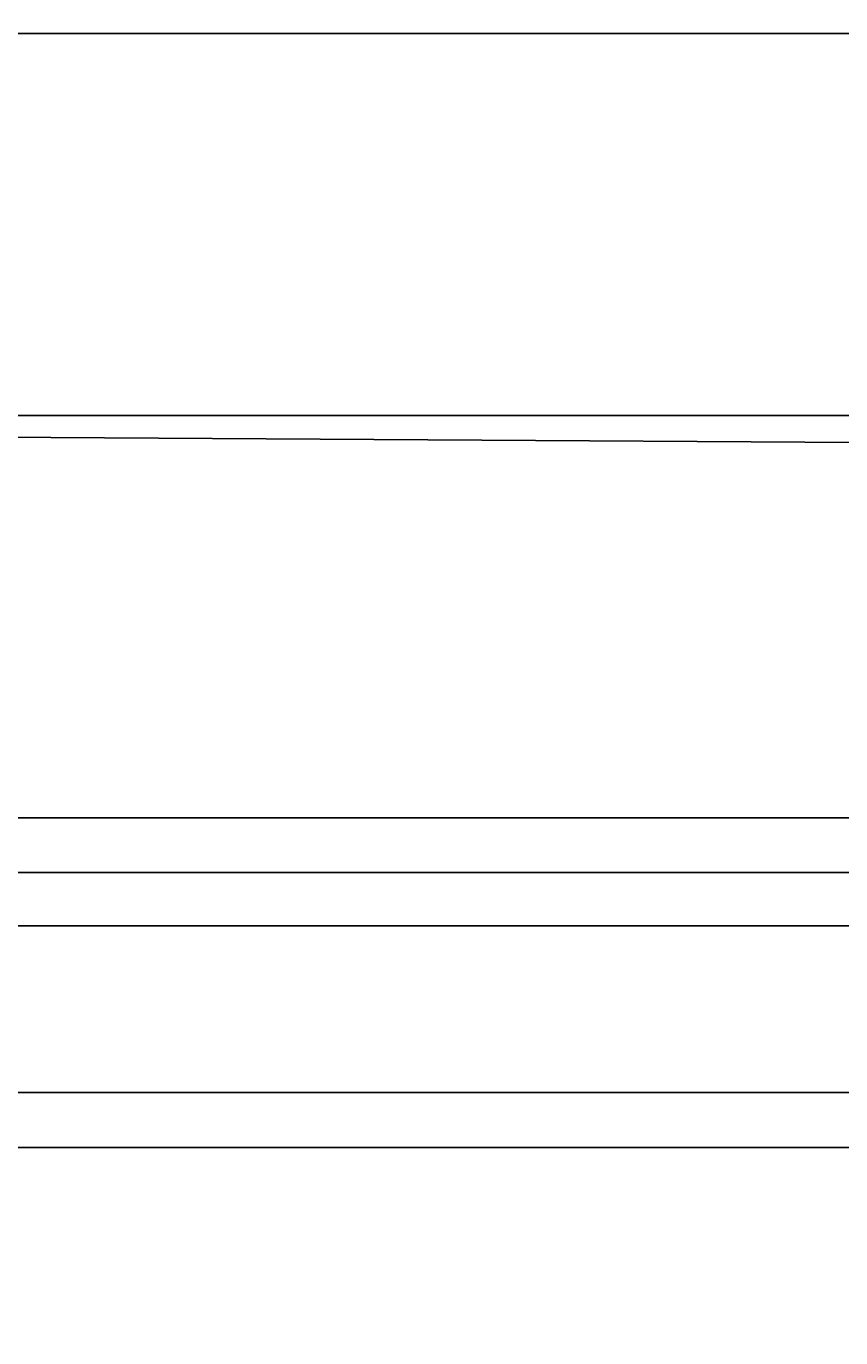
# Model space of a CAD drawing. Units: inches. Extents: x 35362 to 73946, y 43607 to 67532.
# Tile 8 of 134: x 40793 to 42029, y 46919 to 48909. Entities that reach past the tile are written whole.
import ezdxf

# ---------------------------------------------------------------- set-up
doc = ezdxf.new("R2010")
doc.units = ezdxf.units.IN
doc.header["$MEASUREMENT"] = 0
doc.layers.add('A-ANNO-DIMS', color=2, linetype='Continuous', lineweight=18)
doc.layers.add('E-WIRE', color=3, linetype='Continuous', lineweight=25)
doc.styles.get("Standard").update_dxf_attribs({"font": 'arial.ttf'})
doc.dimstyles.get("Standard").update_dxf_attribs({"dimtxt": 0.18, "dimasz": 0.18, "dimexe": 0.18, "dimexo": 0.0625, "dimgap": 0.09, "dimtad": 0, "dimtih": 1, "dimtoh": 1, "dimdec": 4, "dimzin": 0, "dimdsep": 46, "dimtxsty": 'Standard', "dimcen": 0.09, "dimadec": 0, "dimazin": 0, "dimtfac": 1, "dimtdec": 4, "dimtofl": 0, "dimtmove": 0, "dimatfit": 3, "dimfxl": 1, "dimtolj": 1, "dimtzin": 0, "dimarcsym": 0})

# ---------------------------------------------------------------- blocks, each defined once
blk = doc.blocks.new('*D43')
at = {"layer": 'A-ANNO-DIMS', "color": 0, "lineweight": -2, "transparency": 16777216}
for p, q in [((62004.7, 47625.2), (35361.8, 47625.2)), ((35361.9, 47625), (35361.9, 47416.9)), ((35361.9, 47208.4), (35361.9, 47416.5)), ((62004.7, 47208.2), (35361.8, 47208.2))]:
    blk.add_line(p, q, dxfattribs=at)
at = {"layer": 'A-ANNO-DIMS', "color": 0, "transparency": 16777216}
for points in [[(35361.9, 47625), (35362, 47625), (35361.9, 47625.2)], [(35361.9, 47208.4), (35362, 47208.4), (35361.9, 47208.2)]]:
    blk.add_solid(points, dxfattribs=at)
at = {"layer": 'Defpoints', "color": 0, "transparency": 16777216}
for p in [(62004.7, 47625.2), (35361.9, 47208.2), (62004.7, 47208.2)]:
    blk.add_point(p, dxfattribs=at)
at = {"layer": 'A-ANNO-DIMS', "color": 0, "transparency": 16777216, "insert": (35361.9, 47416.7), "char_height": 0.18, "attachment_point": 5}
blk.add_mtext('\\A1;416.9', dxfattribs=at)
blk = doc.blocks.new('*D67')
at = {"layer": 'A-ANNO-DIMS', "color": 0, "lineweight": -2, "transparency": 16777216}
for p, q in [((56873.5, 53351.5), (35361.8, 53351.5)), ((35361.9, 53351.3), (35361.9, 49400.9)), ((35361.9, 45450.1), (35361.9, 49400.5)), ((53793.6, 45449.9), (35361.8, 45449.9))]:
    blk.add_line(p, q, dxfattribs=at)
at = {"layer": 'A-ANNO-DIMS', "color": 0, "transparency": 16777216}
for points in [[(35361.9, 53351.3), (35362, 53351.3), (35361.9, 53351.5)], [(35361.9, 45450.1), (35362, 45450.1), (35361.9, 45449.9)]]:
    blk.add_solid(points, dxfattribs=at)
at = {"layer": 'Defpoints', "color": 0, "transparency": 16777216}
for p in [(35361.9, 53351.5), (56873.6, 53351.5), (53793.6, 45449.9)]:
    blk.add_point(p, dxfattribs=at)
at = {"layer": 'A-ANNO-DIMS', "color": 0, "transparency": 16777216, "insert": (35361.9, 49400.7), "char_height": 0.18, "attachment_point": 5}
blk.add_mtext('\\A1;7901.6', dxfattribs=at)
blk = doc.blocks.new('*D87')
at = {"layer": 'A-ANNO-DIMS', "color": 0, "lineweight": -2, "transparency": 16777216}
for p, q in [((52362.5, 48318.3), (35361.8, 48318.3)), ((35361.9, 48318.1), (35361.9, 47931.4)), ((35361.9, 47544.3), (35361.9, 47931)), ((52362.5, 47544.1), (35361.8, 47544.1))]:
    blk.add_line(p, q, dxfattribs=at)
at = {"layer": 'A-ANNO-DIMS', "color": 0, "transparency": 16777216}
for points in [[(35361.9, 48318.1), (35362, 48318.1), (35361.9, 48318.3)], [(35361.9, 47544.3), (35362, 47544.3), (35361.9, 47544.1)]]:
    blk.add_solid(points, dxfattribs=at)
at = {"layer": 'Defpoints', "color": 0, "transparency": 16777216}
for p in [(35361.9, 48318.3), (52362.6, 48318.3), (52362.6, 47544.1)]:
    blk.add_point(p, dxfattribs=at)
at = {"layer": 'A-ANNO-DIMS', "color": 0, "transparency": 16777216, "insert": (35361.9, 47931.2), "char_height": 0.18, "attachment_point": 5}
blk.add_mtext('\\A1;774.1', dxfattribs=at)
blk = doc.blocks.new('*D89')
at = {"layer": 'A-ANNO-DIMS', "color": 0, "lineweight": -2, "transparency": 16777216}
for p, q in [((53707.7, 48897.7), (35361.8, 48897.7)), ((35361.9, 48897.6), (35361.9, 48303.2)), ((35361.9, 47708.4), (35361.9, 48302.8)), ((53707.7, 47708.2), (35361.8, 47708.2))]:
    blk.add_line(p, q, dxfattribs=at)
at = {"layer": 'A-ANNO-DIMS', "color": 0, "transparency": 16777216}
for points in [[(35361.9, 48897.6), (35362, 48897.6), (35361.9, 48897.7)], [(35361.9, 47708.4), (35362, 47708.4), (35361.9, 47708.2)]]:
    blk.add_solid(points, dxfattribs=at)
at = {"layer": 'Defpoints', "color": 0, "transparency": 16777216}
for p in [(53707.8, 48897.7), (35361.9, 47708.2), (53707.8, 47708.2)]:
    blk.add_point(p, dxfattribs=at)
at = {"layer": 'A-ANNO-DIMS', "color": 0, "transparency": 16777216, "insert": (35361.9, 48303), "char_height": 0.18, "attachment_point": 5}
blk.add_mtext('\\A1;1189.5', dxfattribs=at)
blk = doc.blocks.new('*D90')
at = {"layer": 'A-ANNO-DIMS', "color": 0, "lineweight": -2, "transparency": 16777216}
for p, q in [((53707.7, 47291.3), (35361.8, 47291.3)), ((35361.9, 47291.1), (35361.9, 46710.3)), ((35361.9, 46129.1), (35361.9, 46709.9)), ((53793.6, 46128.9), (35361.8, 46128.9))]:
    blk.add_line(p, q, dxfattribs=at)
at = {"layer": 'A-ANNO-DIMS', "color": 0, "transparency": 16777216}
for points in [[(35361.9, 47291.1), (35362, 47291.1), (35361.9, 47291.3)], [(35361.9, 46129.1), (35362, 46129.1), (35361.9, 46128.9)]]:
    blk.add_solid(points, dxfattribs=at)
at = {"layer": 'Defpoints', "color": 0, "transparency": 16777216}
for p in [(53707.8, 47291.3), (35361.9, 46128.9), (53793.6, 46128.9)]:
    blk.add_point(p, dxfattribs=at)
at = {"layer": 'A-ANNO-DIMS', "color": 0, "transparency": 16777216, "insert": (35361.9, 46710.1), "char_height": 0.18, "attachment_point": 5}
blk.add_mtext('\\A1;1162.4', dxfattribs=at)

msp = doc.modelspace()

# ---------------------------------------------------------------- linework, layer by layer
at = {"layer": 'E-WIRE'}
msp.add_line((39894.84, 48290.562), (42056.036, 48277.555), dxfattribs=at)

# ---------------------------------------------------------------- dimensions: what is measured, and where the dimension line sits
at = {"layer": 'A-ANNO-DIMS'}
for base, p1, p2, picture, middle in [((35361.949, 53351.529), (53793.638, 45449.894), (56873.602, 53351.529), '*D67', (35361.949, 49400.712)), ((35361.949, 47708.216), (53707.781, 48897.738), (53707.781, 47708.216), '*D89', (35361.949, 48302.977)), ((35361.949, 48318.269), (52362.557, 47544.134), (52362.557, 48318.269), '*D87', (35361.949, 47931.201)), ((35361.949, 47208.25), (62004.728, 47625.181), (62004.728, 47208.25), '*D43', (35361.949, 47416.715)), ((35361.949, 46128.878), (53707.781, 47291.285), (53793.638, 46128.878), '*D90', (35361.949, 46710.081))]:
    dim = msp.add_linear_dim(base=base, p1=p1, p2=p2, angle=90, dimstyle='Standard', override={"dimdec": 1, "dimlfac": 1, "dimrnd": 0, "dimzin": 0, "dimdsep": 46, "dimlunit": 2}, dxfattribs=at)
    dim.commit()
    dim.dimension.update_dxf_attribs({"geometry": picture, "text_midpoint": middle})

doc.saveas('drawing.dxf')
